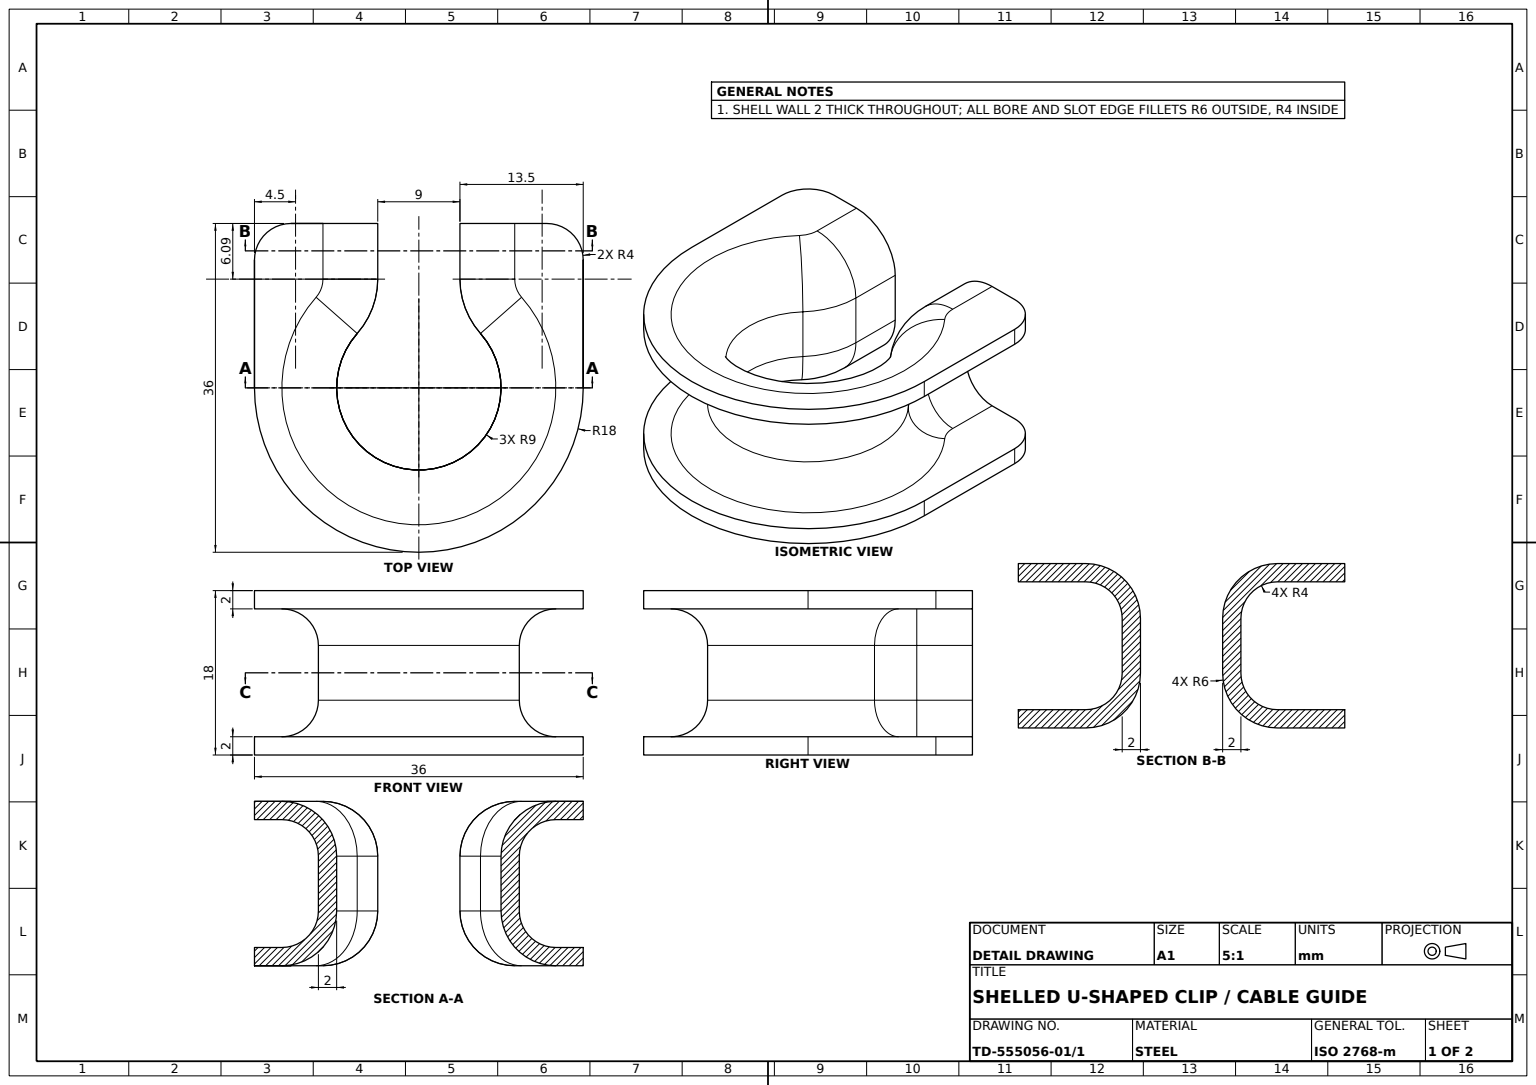
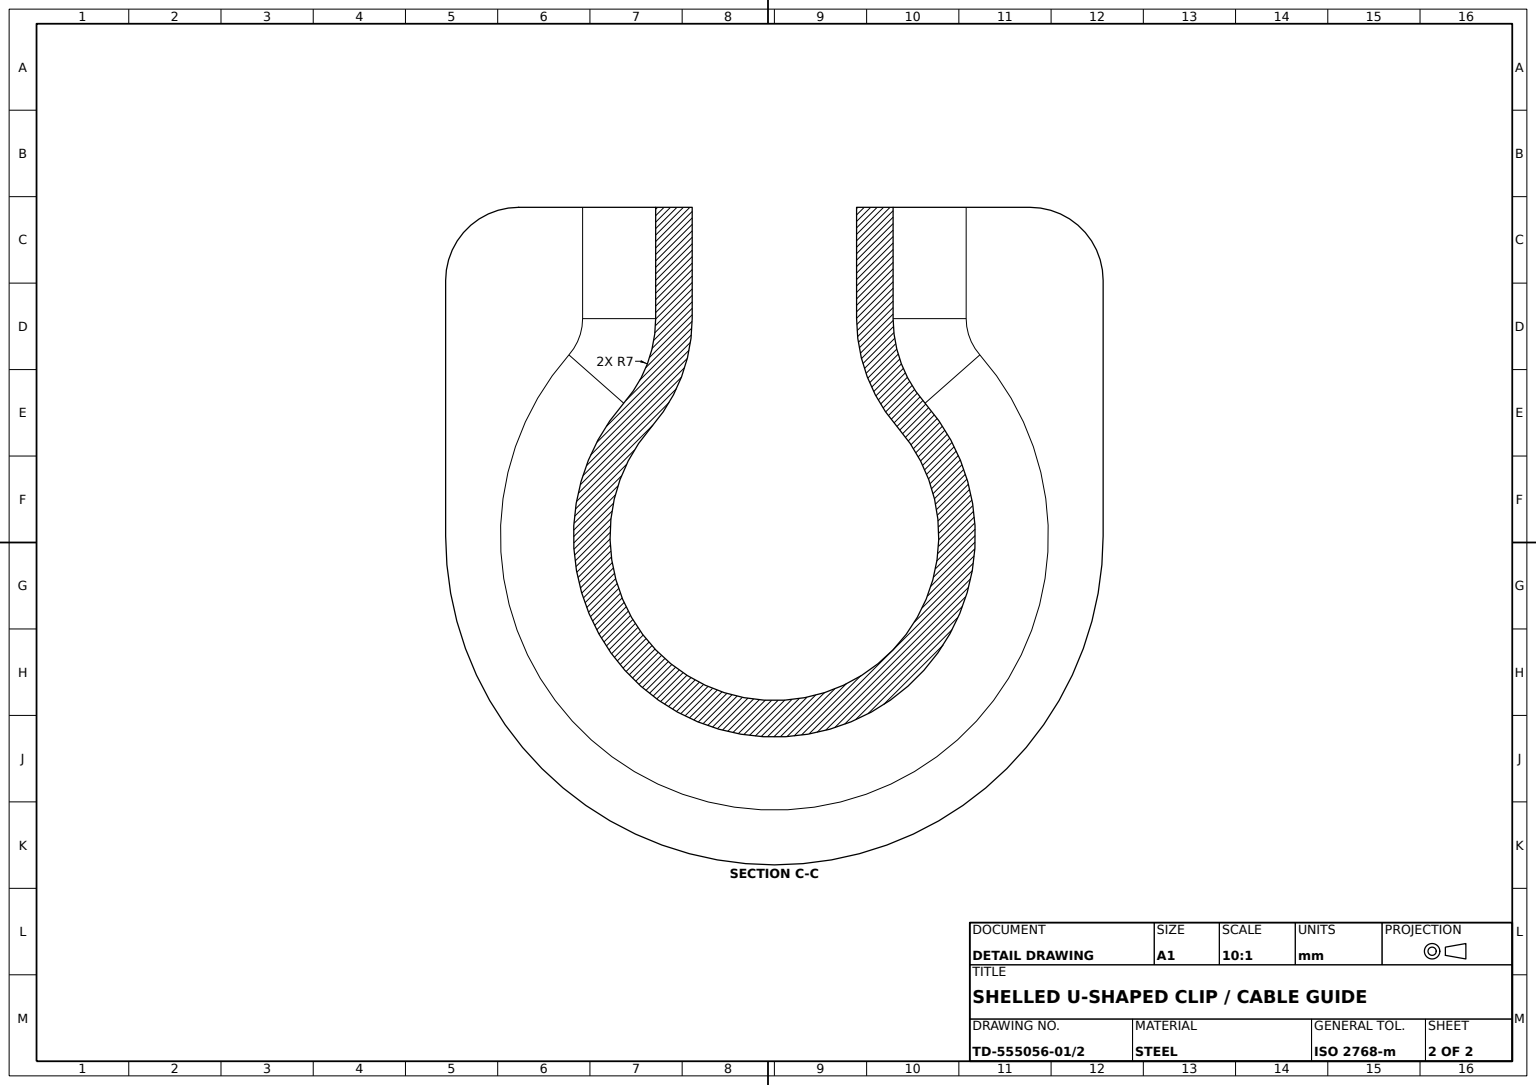
from build123d import *

# Parameters (mm, degrees)
CLIP_BODY_EXTRUDE_18MM_DEPTH = 9
EDGE_FILLETS_R6_R            = 6
SHELL_WALL_2MM_T             = -2


with BuildPart() as part:
    # Clip Profile Sketch → Clip Body Extrude 18mm (new, symmetric)
    with BuildSketch(Plane(origin=(0, 0, 0), x_dir=(1, 0, 0), z_dir=(0, 1, 0))):
        with BuildLine():
            Line((-14, 18), (-4.5, 18))
            Line((-4.5, 18), (-4.5, 11.9058809))
            ThreePointArc((-4.5, 11.9058809), (-5.08127088, 8.723900384), (-6.75, 5.95294045))
            ThreePointArc((-6.75, 5.95294045), (0, -9), (6.75, 5.95294045))
            ThreePointArc((6.75, 5.95294045), (5.08127088, 8.723900384), (4.5, 11.9058809))
            Line((4.5, 11.9058809), (4.5, 18))
            Line((4.5, 18), (14, 18))
            ThreePointArc((14, 18), (16.828427125, 16.828427125), (18, 14))
            Line((18, 14), (18, 0))
            ThreePointArc((18, 0), (0, -18), (-18, 0))
            Line((-18, 0), (-18, 14))
            ThreePointArc((-18, 14), (-16.828427125, 16.828427125), (-14, 18))
        make_face()
    extrude(amount=CLIP_BODY_EXTRUDE_18MM_DEPTH, both=True)

    # Edge Fillets R6
    edge_fillets_r6_edges = [part.edges().sort_by_distance(p)[0] for p in [
        (0, -9, 9),
        (5.08127088, -9, -8.723900384),
        (4.5, -9, -14.95294045),
        (-4.5, -9, -14.95294045),
        (-5.08127088, -9, -8.723900384),
        (4.5, 9, -14.95294045),
        (5.08127088, 9, -8.723900384),
        (0, 9, 9),
        (-5.08127088, 9, -8.723900384),
        (-4.5, 9, -14.95294045),
    ]]
    fillet(edge_fillets_r6_edges, radius=EDGE_FILLETS_R6_R)

    # Shell Wall 2mm
    shell_wall_2mm_openings = [part.faces().sort_by_distance(p)[0] for p in [
        (-9.588709649, 0, -18),
        (-16.828427125, 0, -16.828427125),
        (-18, 0, -7),
        (0, 0, 18),
        (18, 0, -7),
        (16.828427125, 0, -16.828427125),
        (9.588709649, 0, -18),
    ]]
    offset(amount=SHELL_WALL_2MM_T, openings=shell_wall_2mm_openings, kind=Kind.INTERSECTION)


solid = part.part
